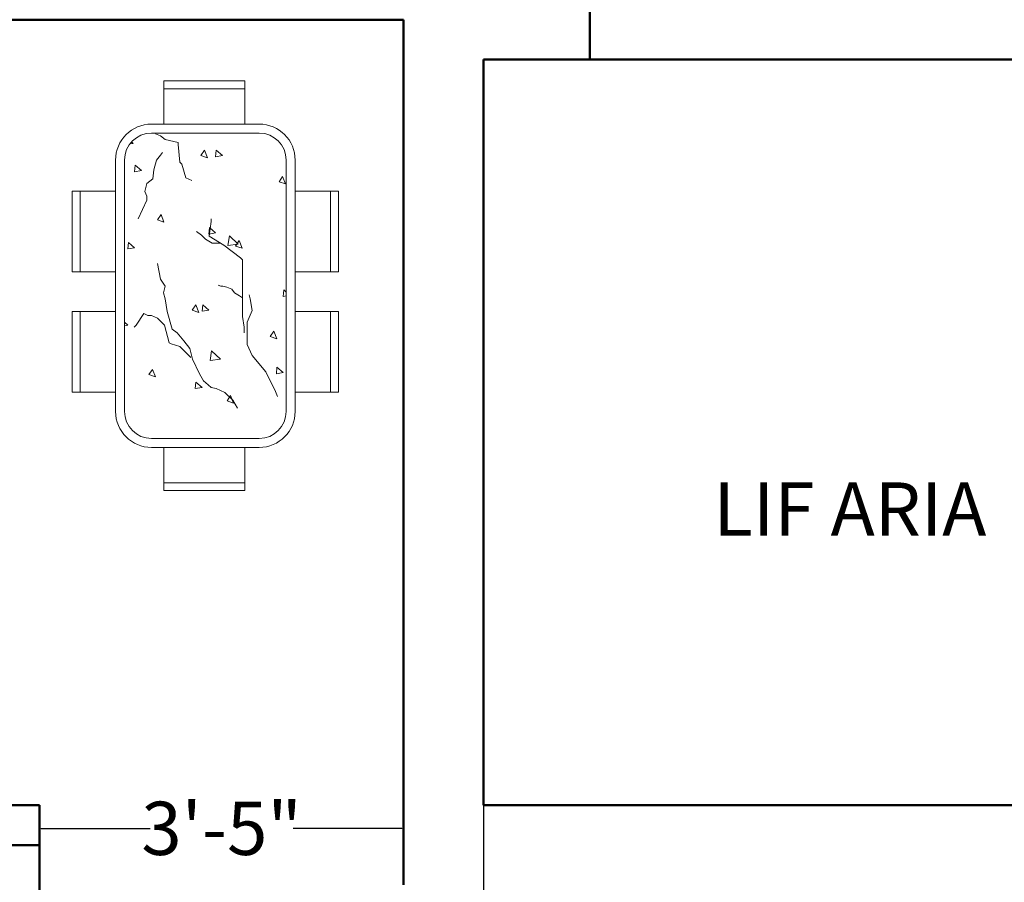
# Model space of a CAD drawing. Units: inches. Extents: x -173 to 545, y -746 to 104.
# Tile 14 of 32: x 168 to 278, y -561 to -463. Entities that reach past the tile are written whole.
import ezdxf

# ---------------------------------------------------------------- set-up
doc = ezdxf.new("R2010")
doc.units = ezdxf.units.IN
doc.header["$MEASUREMENT"] = 0
for name, color, linetype, lineweight in [('A-ANNO-DIMS', 2, 'Continuous', 18), ('A-AREA-IDEN', 7, 'Continuous', 18), ('A-FURN', 8, 'Continuous', 18), ('A-WALL', 7, 'Continuous', 50)]:
    doc.layers.add(name, color=color, linetype=linetype, lineweight=lineweight)
doc.styles.get("Standard").update_dxf_attribs({"font": 'arial.ttf'})
doc.dimstyles.get("Standard").update_dxf_attribs({"dimtxt": 0.18, "dimasz": 0.18, "dimexe": 0.18, "dimexo": 0.0625, "dimgap": 0.09, "dimtad": 0, "dimtih": 1, "dimtoh": 1, "dimdec": 0, "dimzin": 0, "dimdsep": 46, "dimlunit": 3, "dimtxsty": 'Standard', "dimcen": 0.09, "dimadec": 0, "dimazin": 0, "dimtfac": 1, "dimtdec": 0, "dimtofl": 0, "dimtmove": 0, "dimatfit": 3, "dimfxl": 1, "dimtolj": 1, "dimtzin": 0, "dimarcsym": 0})

# ---------------------------------------------------------------- blocks, each defined once
blk = doc.blocks.new('*D15')
at = {"layer": 'A-ANNO-DIMS', "color": 0, "lineweight": -2, "transparency": 16777216}
for p, q in [((169.8, -551.92), (169.8, -554.66)), ((210.8, -551.92), (210.8, -554.66)), ((169.98, -554.48), (182.24, -554.48)), ((210.62, -554.48), (198.36, -554.48))]:
    blk.add_line(p, q, dxfattribs=at)
at = {"layer": 'A-ANNO-DIMS', "color": 0, "transparency": 16777216}
for points in [[(169.98, -554.45), (169.98, -554.51), (169.8, -554.48)], [(210.62, -554.45), (210.62, -554.51), (210.8, -554.48)]]:
    blk.add_solid(points, dxfattribs=at)
at = {"layer": 'Defpoints', "color": 0, "transparency": 16777216}
for p in [(169.8, -551.86), (210.8, -551.86), (210.8, -554.48)]:
    blk.add_point(p, dxfattribs=at)
at = {"layer": 'A-ANNO-DIMS', "color": 0, "transparency": 16777216, "insert": (190.3, -554.48), "char_height": 6, "attachment_point": 5}
blk.add_mtext('\\A1;3\'-5"', dxfattribs=at)
blk = doc.blocks.new('DINING-TABLE-SIX')
for p, q in [((19.42, 46.17), (10.32, 46.17)), ((10.32, 46.17), (10.32, 41.3)), ((19.42, 41.3), (19.42, 46.17)), ((10.32, 45.28), (19.42, 45.28)), ((21.06, 41.3), (8.92, 41.3)), ((8.92, 40.29), (21.06, 40.29)), ((9.38, 40.21), (9.93, 39.99)), ((9.93, 39.99), (10.48, 39.55)), ((6.49, 39.07), (6.86, 39.11)), ((6.68, 39.29), (6.86, 39.11)), ((10.48, 39.55), (11.91, 39.22)), ((11.91, 39.22), (11.91, 39)), ((11.91, 39), (12.13, 37.02)), ((9.5, 37.24), (9.94, 37.79)), ((9.94, 37.79), (10.16, 38.12)), ((14.89, 38.37), (14.48, 37.76)), ((14.48, 37.76), (15.22, 37.52)), ((14.89, 38.37), (15.22, 37.52)), ((16.21, 38.35), (16.15, 37.62)), ((16.15, 37.62), (16.91, 37.76)), ((16.21, 38.35), (16.91, 37.76)), ((4.88, 37.25), (4.88, 8.92)), ((5.89, 8.92), (5.89, 37.25)), ((7.08, 36.66), (7.02, 35.94)), ((7.08, 36.66), (7.78, 36.08)), ((9.17, 36.14), (9.5, 37.24)), ((12.13, 37.02), (12.35, 36.8)), ((12.35, 36.8), (12.79, 35.26)), ((24.1, 37.25), (24.1, 8.92)), ((25.11, 8.92), (25.11, 37.25)), ((7.02, 35.94), (7.78, 36.08)), ((9.06, 35.15), (9.17, 36.14)), ((8.18, 33.72), (8.4, 34.6)), ((8.4, 34.6), (9.06, 35.15)), ((12.79, 35.26), (13.45, 34.93)), ((23.69, 35.41), (23.29, 34.81)), ((23.29, 34.81), (24.02, 34.56)), ((23.69, 35.41), (24.02, 34.56)), ((4.88, 33.75), (0, 33.75)), ((0, 33.75), (0, 24.64)), ((0.89, 24.64), (0.89, 33.75)), ((8.4, 33.17), (8.18, 33.72)), ((25.11, 33.75), (29.99, 33.75)), ((29.1, 24.64), (29.1, 33.75)), ((29.99, 33.75), (29.99, 24.64)), ((7.41, 30.64), (8.4, 32.73)), ((8.4, 32.73), (8.4, 33.17)), ((10, 31.12), (9.6, 30.52)), ((10, 31.12), (10.33, 30.27)), ((9.59, 30.52), (10.33, 30.27)), ((15.43, 28.66), (15.65, 30.31)), ((15.65, 30.31), (15.65, 30.64)), ((14.55, 28.77), (14, 29.21)), ((15.45, 29.64), (15.39, 28.91)), ((15.39, 28.91), (16.15, 29.05)), ((15.45, 29.64), (16.15, 29.05)), ((6.32, 27.95), (6.25, 27.23)), ((6.32, 27.95), (7.02, 27.37)), ((14.99, 28.33), (14.55, 28.77)), ((15.76, 27.89), (14.99, 28.33)), ((17.08, 27.67), (15.43, 28.66)), ((16.75, 27.89), (15.76, 27.89)), ((17.7, 28.71), (17.54, 27.63)), ((17.54, 27.63), (18.69, 27.77)), ((17.7, 28.71), (18.69, 27.77)), ((18.81, 28.17), (18.4, 27.56)), ((18.81, 28.17), (19.13, 27.32)), ((6.25, 27.23), (7.02, 27.37)), ((18.94, 26.24), (17.08, 27.67)), ((18.4, 27.56), (19.13, 27.32)), ((9.93, 23.82), (9.6, 25.58)), ((19.16, 26.02), (18.94, 26.24)), ((19.16, 19.64), (19.16, 26.02)), ((0, 24.64), (4.88, 24.64)), ((29.99, 24.64), (25.11, 24.64)), ((10.48, 23.05), (9.93, 23.82)), ((10.26, 22.28), (10.48, 23.05)), ((10.48, 21.62), (10.26, 22.28)), ((16.75, 23.05), (16.42, 23.16)), ((16.97, 23.05), (16.75, 23.05)), ((17.41, 22.94), (16.97, 23.05)), ((17.96, 22.72), (17.41, 22.94)), ((18.29, 22.28), (17.96, 22.72)), ((18.84, 21.95), (18.29, 22.28)), ((23.82, 22.62), (23.76, 21.89)), ((23.82, 22.62), (24.1, 22.38)), ((10.7, 20.19), (10.48, 21.62)), ((19.17, 21.73), (18.84, 21.95)), ((20.04, 21.62), (19.93, 22.06)), ((20.26, 20.3), (20.04, 21.62)), ((23.76, 21.89), (24.1, 21.95)), ((4.88, 20.19), (0, 20.19)), ((0, 20.19), (0, 11.09)), ((0.89, 11.09), (0.89, 20.19)), ((11.25, 18.21), (10.7, 20.19)), ((13.92, 20.92), (13.51, 20.32)), ((13.51, 20.32), (14.24, 20.07)), ((13.92, 20.92), (14.24, 20.07)), ((14.69, 20.93), (14.62, 20.21)), ((14.62, 20.21), (15.39, 20.35)), ((14.69, 20.93), (15.39, 20.35)), ((19.71, 18.98), (20.26, 20.3)), ((25.11, 20.19), (29.99, 20.19)), ((29.1, 11.09), (29.1, 20.19)), ((29.99, 20.19), (29.99, 11.09)), ((5.89, 18.97), (6.25, 18.66)), ((8.07, 19.97), (7.19, 18.65)), ((8.51, 19.75), (8.07, 19.97)), ((8.94, 19.75), (8.51, 19.75)), ((9.6, 19.42), (8.94, 19.75)), ((10.37, 18.65), (9.6, 19.42)), ((19.38, 18.43), (19.16, 19.64)), ((19.71, 16.45), (19.71, 18.98)), ((5.89, 18.59), (6.25, 18.66)), ((7.19, 18.65), (6.97, 18.43)), ((10.92, 16.67), (10.37, 18.65)), ((11.8, 17.77), (11.25, 18.21)), ((12.57, 16.89), (11.8, 17.77)), ((19.38, 17.77), (19.38, 18.43)), ((22.72, 17.97), (22.31, 17.36)), ((22.72, 17.97), (23.05, 17.12)), ((11.14, 16.56), (10.92, 16.67)), ((13.23, 16.01), (12.57, 16.89)), ((22.31, 17.36), (23.05, 17.12)), ((12.13, 16.23), (11.14, 16.56)), ((12.9, 15.46), (12.13, 16.23)), ((13.56, 14.8), (13.23, 16.01)), ((15.69, 15.75), (15.53, 14.68)), ((15.69, 15.75), (16.68, 14.81)), ((20.26, 15.24), (19.71, 16.45)), ((13.34, 15.02), (12.9, 15.46)), ((14.33, 13.15), (13.56, 14.8)), ((15.53, 14.68), (16.68, 14.81)), ((21.8, 13.37), (20.26, 15.24)), ((9.03, 13.67), (8.62, 13.07)), ((9.03, 13.67), (9.36, 12.82)), ((22.9, 11.17), (21.8, 13.37)), ((23.06, 13.91), (22.99, 13.18)), ((22.99, 13.18), (23.76, 13.32)), ((23.06, 13.91), (23.76, 13.32)), ((8.62, 13.07), (9.36, 12.82)), ((13.93, 12.22), (13.86, 11.5)), ((13.93, 12.22), (14.62, 11.64)), ((14.77, 12.38), (14.33, 13.15)), ((15.32, 11.94), (14.77, 12.38)), ((13.86, 11.5), (14.62, 11.64)), ((15.65, 11.61), (15.32, 11.94)), ((16.2, 11.5), (15.65, 11.61)), ((17.19, 11.06), (16.2, 11.5)), ((23.12, 10.62), (22.9, 11.17)), ((0, 11.09), (4.88, 11.09)), ((18.07, 10.18), (17.19, 11.06)), ((17.83, 10.72), (17.43, 10.11)), ((17.43, 10.11), (18.16, 9.87)), ((17.83, 10.72), (18.16, 9.87)), ((18.61, 9.3), (18.07, 10.18)), ((29.99, 11.09), (25.11, 11.09)), ((21.06, 5.89), (8.92, 5.89)), ((8.92, 4.88), (21.06, 4.88)), ((10.32, 4.88), (10.32, 0)), ((19.42, 0), (19.42, 4.88)), ((19.42, 0.89), (10.32, 0.89)), ((10.32, 0), (19.42, 0))]:
    blk.add_line(p, q)
for centre, radius, start, end in [((8.92, 37.25), 4.05, 90, 180), ((21.06, 37.25), 4.05, 0, 90), ((8.92, 37.25), 3.04, 90, 180), ((21.06, 37.25), 3.04, 0, 90), ((8.92, 8.92), 4.05, 180, 270), ((8.92, 8.92), 3.04, 180, 270), ((21.06, 8.92), 3.04, 270, 0), ((21.06, 8.92), 4.05, 270, 0)]:
    blk.add_arc(centre, radius, start, end)
blk = doc.blocks.new('*D81')
at = {"layer": 'A-ANNO-DIMS', "color": 0, "lineweight": -2, "transparency": 16777216}
for p, q in [((219.8, -551.92), (219.8, -740.64)), ((306.3, -551.92), (306.3, -740.64)), ((219.98, -740.46), (262.51, -740.46)), ((306.12, -740.46), (263.59, -740.46))]:
    blk.add_line(p, q, dxfattribs=at)
at = {"layer": 'A-ANNO-DIMS', "color": 0, "transparency": 16777216}
for points in [[(219.98, -740.43), (219.98, -740.49), (219.8, -740.46)], [(306.12, -740.43), (306.12, -740.49), (306.3, -740.46)]]:
    blk.add_solid(points, dxfattribs=at)
at = {"layer": 'Defpoints', "color": 0, "transparency": 16777216}
for p in [(219.8, -551.86), (306.3, -551.86), (306.3, -740.46)]:
    blk.add_point(p, dxfattribs=at)
at = {"layer": 'A-ANNO-DIMS', "color": 0, "transparency": 16777216, "insert": (263.05, -740.46), "char_height": 0.18, "attachment_point": 5}
blk.add_mtext('\\A1;7\'-2 1/2"', dxfattribs=at)
blk = doc.blocks.new('*D82')
at = {"layer": 'A-ANNO-DIMS', "color": 0, "lineweight": -2, "transparency": 16777216}
for p, q in [((219.86, -467.86), (545.08, -467.86)), ((544.9, -468.04), (544.9, -509.68)), ((544.9, -551.68), (544.9, -510.04)), ((219.86, -551.86), (545.08, -551.86))]:
    blk.add_line(p, q, dxfattribs=at)
at = {"layer": 'A-ANNO-DIMS', "color": 0, "transparency": 16777216}
for points in [[(544.87, -468.04), (544.93, -468.04), (544.9, -467.86)], [(544.87, -551.68), (544.93, -551.68), (544.9, -551.86)]]:
    blk.add_solid(points, dxfattribs=at)
at = {"layer": 'Defpoints', "color": 0, "transparency": 16777216}
for p in [(219.8, -467.86), (219.8, -551.86), (544.9, -551.86)]:
    blk.add_point(p, dxfattribs=at)
at = {"layer": 'A-ANNO-DIMS', "color": 0, "transparency": 16777216, "insert": (544.9, -509.86), "char_height": 0.18, "attachment_point": 5}
blk.add_mtext('\\A1;7\'-0"', dxfattribs=at)

msp = doc.modelspace()

# ---------------------------------------------------------------- linework, layer by layer
at = {"layer": 'A-WALL'}
for p, q in [((231.8, -458.86), (231.8, -467.86)), ((156.8, -463.36), (210.8, -463.36)), ((210.8, -463.36), (210.8, -560.86)), ((219.8, -467.86), (306.3, -467.86)), ((219.8, -467.86), (219.8, -551.86)), ((85.8, -551.86), (169.8, -551.86)), ((169.8, -551.86), (169.8, -688.36)), ((219.8, -551.86), (306.3, -551.86)), ((33.3, -556.36), (169.8, -556.36))]:
    msp.add_line(p, q, dxfattribs=at)

# ---------------------------------------------------------------- block references
at = {"layer": 'A-FURN'}
msp.add_blockref('DINING-TABLE-SIX', (173.48, -516.43), dxfattribs=at)

# ---------------------------------------------------------------- texts
at = {"layer": 'A-AREA-IDEN', "insert": (245.72, -515.5), "char_height": 6, "attachment_point": 1}
msp.add_mtext('LIF ARIA', dxfattribs=at)

# ---------------------------------------------------------------- dimensions: what is measured, and where the dimension line sits
at = {"layer": 'A-ANNO-DIMS'}
dim = msp.add_linear_dim(base=(544.9, -551.86), p1=(219.8, -467.86), p2=(219.8, -551.86), angle=90, dimstyle='Standard', override={"dimdec": 1, "dimlfac": 1, "dimrnd": 0, "dimzin": 1, "dimdsep": 46, "dimlunit": 4, "dimfrac": 2}, dxfattribs=at)
dim.commit()
dim.dimension.update_dxf_attribs({"geometry": '*D82', "text_midpoint": (544.9, -509.86)})
for base, p1, p2, override, picture, middle in [((210.8, -554.48), (169.8, -551.86), (210.8, -551.86), {"dimtxt": 6, "dimclrd": 0, "dimclre": 0, "dimclrt": 0}, '*D15', (190.3, -554.48)), ((306.3, -740.46), (219.8, -551.86), (306.3, -551.86), {"dimdec": 1, "dimlfac": 1, "dimrnd": 0, "dimzin": 1, "dimdsep": 46, "dimlunit": 4, "dimfrac": 2}, '*D81', (263.05, -740.46))]:
    dim = msp.add_linear_dim(base=base, p1=p1, p2=p2, dimstyle='Standard', override=override, dxfattribs=at)
    dim.commit()
    dim.dimension.update_dxf_attribs({"geometry": picture, "text_midpoint": middle})

doc.saveas('drawing.dxf')
